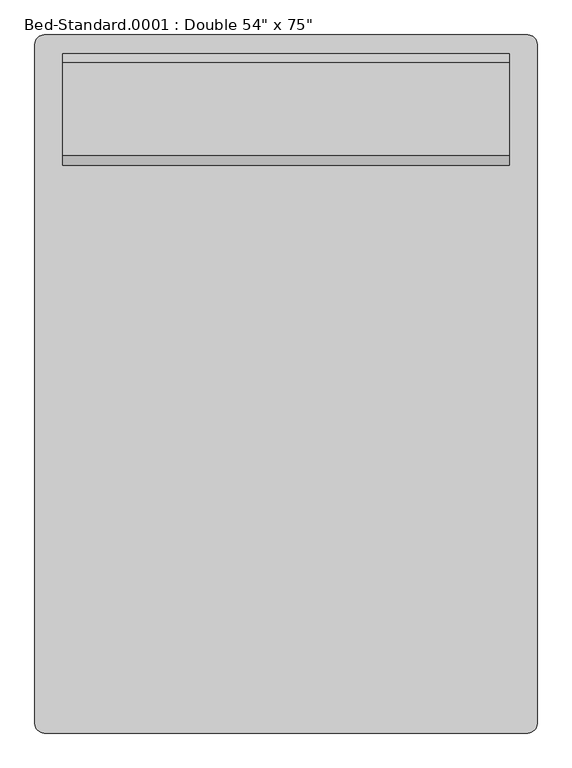
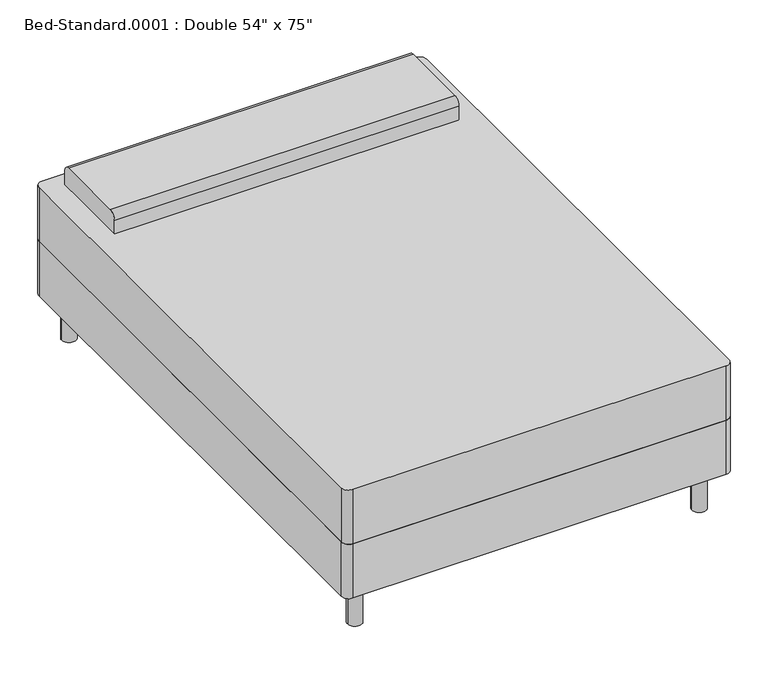
"""IFC4 building model written with IfcOpenShell, lengths in millimetres: furniture geometry."""

from ifc_helpers import new_model, si_unit, point, frame, frame_2d, origin, origin_with_axes, place, context, project, spatial, polyline, circle_curve, trimmed, segment, composite_curve, outline, extrude, source, transform, mapped, element, save


def furniture_0253826f(model_context):
    return source(origin(), model_context, "Body", "SweptSolid", [
        extrude(outline(composite_curve([segment(polyline([(-414.3114754, -972.695082), (-414.3114754, 881.504918)]), True, "CONTINUOUS"), segment(trimmed(circle_curve(frame_2d((-388.9114754, 881.504918)), 25.4), [point((-414.3114754, 881.504918))], [point((-388.9114754, 906.904918))], False, "CARTESIAN"), True, "CONTINUOUS"), segment(polyline([(-388.9114754, 906.904918), (931.8885246, 906.904918)]), True, "CONTINUOUS"), segment(trimmed(circle_curve(frame_2d((931.8885246, 881.504918)), 25.4), [point((931.8885246, 906.904918))], [point((957.2885246, 881.504918))], False, "CARTESIAN"), True, "CONTINUOUS"), segment(polyline([(957.2885246, 881.504918), (957.2885246, -972.695082)]), True, "CONTINUOUS"), segment(trimmed(circle_curve(frame_2d((931.8885246, -972.695082)), 25.4), [point((957.2885246, -972.695082))], [point((931.8885246, -998.095082))], False, "CARTESIAN"), True, "CONTINUOUS"), segment(polyline([(931.8885246, -998.095082), (-388.9114754, -998.095082)]), True, "CONTINUOUS"), segment(trimmed(circle_curve(frame_2d((-388.9114754, -972.695082)), 25.4), [point((-388.9114754, -998.095082))], [point((-414.3114754, -972.695082))], False, "CARTESIAN"), True, "CONTINUOUS")], self_intersect=False)), frame((0.0, 0.0, 152.4), z_axis=(0.0, 0.0, 1.0), x_axis=(1.0, 0.0, 0.0)), (0.0, 0.0, 1.0), 203.2),
        extrude(outline(composite_curve([segment(polyline([(551.304918, 558.8), (551.304918, 609.6)]), True, "CONTINUOUS"), segment(trimmed(circle_curve(frame_2d((576.704918, 609.6)), 25.4), [point((551.304918, 609.6))], [point((576.704918, 635.0))], False, "CARTESIAN"), True, "CONTINUOUS"), segment(polyline([(576.704918, 635.0), (830.704918, 635.0)]), True, "CONTINUOUS"), segment(trimmed(circle_curve(frame_2d((830.704918, 609.6)), 25.4), [point((830.704918, 635.0))], [point((856.104918, 609.6))], False, "CARTESIAN"), True, "CONTINUOUS"), segment(polyline([(856.104918, 609.6), (856.104918, 558.8), (551.304918, 558.8)]), True, "CONTINUOUS")], self_intersect=False)), frame((-338.1114754, 0.0, 0.0), z_axis=(1.0, 0.0, 0.0), x_axis=(0.0, 1.0, 0.0)), (0.0, 0.0, 1.0), 1219.2),
        extrude(outline(composite_curve([segment(trimmed(circle_curve(frame_2d((-338.1114754, 830.704918)), 25.4), [point((-363.5114754, 830.704918))], [point((-312.7114754, 830.704918))], False, "CARTESIAN"), True, "CONTINUOUS"), segment(trimmed(circle_curve(frame_2d((-338.1114754, 830.704918)), 25.4), [point((-312.7114754, 830.704918))], [point((-363.5114754, 830.704918))], False, "CARTESIAN"), True, "CONTINUOUS")], self_intersect=False)), origin_with_axes(), (0.0, 0.0, 1.0), 152.4),
        extrude(outline(composite_curve([segment(trimmed(circle_curve(frame_2d((881.0885246, 830.704918)), 25.4), [point((855.6885246, 830.704918))], [point((906.4885246, 830.704918))], False, "CARTESIAN"), True, "CONTINUOUS"), segment(trimmed(circle_curve(frame_2d((881.0885246, 830.704918)), 25.4), [point((906.4885246, 830.704918))], [point((855.6885246, 830.704918))], False, "CARTESIAN"), True, "CONTINUOUS")], self_intersect=False)), origin_with_axes(), (0.0, 0.0, 1.0), 152.4),
        extrude(outline(composite_curve([segment(trimmed(circle_curve(frame_2d((881.0885246, -921.895082)), 25.4), [point((855.6885246, -921.895082))], [point((906.4885246, -921.895082))], False, "CARTESIAN"), True, "CONTINUOUS"), segment(trimmed(circle_curve(frame_2d((881.0885246, -921.895082)), 25.4), [point((906.4885246, -921.895082))], [point((855.6885246, -921.895082))], False, "CARTESIAN"), True, "CONTINUOUS")], self_intersect=False)), origin_with_axes(), (0.0, 0.0, 1.0), 152.4),
        extrude(outline(composite_curve([segment(trimmed(circle_curve(frame_2d((-338.1114754, -921.895082)), 25.4), [point((-363.5114754, -921.895082))], [point((-312.7114754, -921.895082))], False, "CARTESIAN"), True, "CONTINUOUS"), segment(trimmed(circle_curve(frame_2d((-338.1114754, -921.895082)), 25.4), [point((-312.7114754, -921.895082))], [point((-363.5114754, -921.895082))], False, "CARTESIAN"), True, "CONTINUOUS")], self_intersect=False)), origin_with_axes(), (0.0, 0.0, 1.0), 152.4),
        extrude(outline(composite_curve([segment(polyline([(-388.9114754, 906.904918), (931.8885246, 906.904918)]), True, "CONTINUOUS"), segment(trimmed(circle_curve(frame_2d((931.8885246, 881.504918)), 25.4), [point((931.8885246, 906.904918))], [point((957.2885246, 881.504918))], False, "CARTESIAN"), True, "CONTINUOUS"), segment(polyline([(957.2885246, 881.504918), (957.2885246, -972.695082)]), True, "CONTINUOUS"), segment(trimmed(circle_curve(frame_2d((931.8885246, -972.695082)), 25.4), [point((957.2885246, -972.695082))], [point((931.8885246, -998.095082))], False, "CARTESIAN"), True, "CONTINUOUS"), segment(polyline([(931.8885246, -998.095082), (-388.9114754, -998.095082)]), True, "CONTINUOUS"), segment(trimmed(circle_curve(frame_2d((-388.9114754, -972.695082)), 25.4), [point((-388.9114754, -998.095082))], [point((-414.3114754, -972.695082))], False, "CARTESIAN"), True, "CONTINUOUS"), segment(polyline([(-414.3114754, -972.695082), (-414.3114754, 881.504918)]), True, "CONTINUOUS"), segment(trimmed(circle_curve(frame_2d((-388.9114754, 881.504918)), 25.4), [point((-414.3114754, 881.504918))], [point((-388.9114754, 906.904918))], False, "CARTESIAN"), True, "CONTINUOUS")], self_intersect=False)), frame((0.0, 0.0, 355.6), z_axis=(0.0, 0.0, 1.0), x_axis=(1.0, 0.0, 0.0)), (0.0, 0.0, 1.0), 203.2),
    ])


if __name__ == "__main__":
    model = new_model("IFC4")
    model_context = context("Model", 3, world=origin())
    ifc_project = project(units=[si_unit("LENGTHUNIT", "METRE", prefix="MILLI")], contexts=[model_context])
    site = spatial("IfcSite", under=ifc_project)
    building = spatial("IfcBuilding", under=site)
    placement = place(None, origin())
    furniture_shape = furniture_0253826f(model_context)
    element("IfcFurniture", 1, ObjectType="Bed-Standard.0001 : Double 54\" x 75\"", at=placement, inside=building, context=model_context, shape_type="MappedRepresentation", body=[
        mapped(furniture_shape, transform((0.0, 0.0, 0.0), x_axis=(1.0, 0.0, 0.0), y_axis=(0.0, 1.0, 0.0), z_axis=(0.0, 0.0, 1.0))),
    ])
    save(model, "model.ifc")

# Revit data of these elements
# Type "Bed-Standard.0001 : Double 54\" x 75\""
#   Assembly Code = "E2020200"
#   Length = 6' - 3"
#   Width = 4' - 6"
#   Leg Material = Steel, Chrome Plated
#   Mattress Material = Linen, White
#   Default Elevation = 0
# Element 1 (IfcFurniture, "Bed-Standard.0001 : Double 54\" x 75\"")
#   Materials on its faces: "Linen, White", "Steel, Chrome Plated"
# Materials
#   "Steel, Chrome Plated": class "Metal", colour RGB 17 17 17, transparency 0, Description = "Chromiuim plated steel", Cost = 0
#   "Linen, White": class "Textile", colour RGB 247 247 239, transparency 0, Description = "Linen, white", Cost = 0
